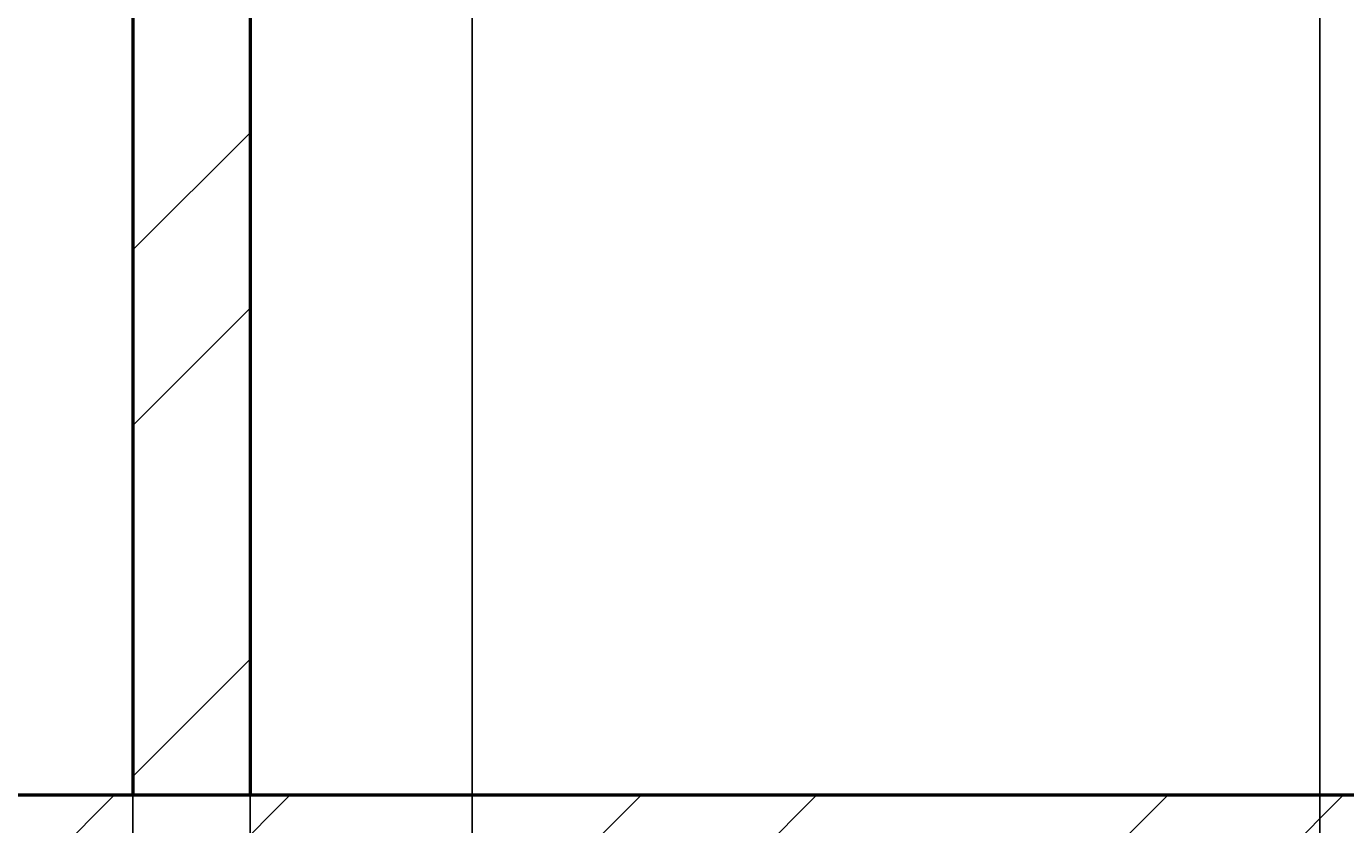
# Model space of a CAD drawing. Units: inches. Extents: x 2812 to 3051, y 1398 to 1659.
# Tile 50 of 65: x 2878 to 2911, y 1559 to 1579. Entities that reach past the tile are written whole.
import ezdxf

# ---------------------------------------------------------------- set-up
doc = ezdxf.new("R2010")
doc.units = ezdxf.units.IN
for name, color, linetype, lineweight in [('A-ANNO-DIMS', 2, 'Continuous', 18), ('S-CONC', 7, 'Continuous', 50), ('S-CONC-PATT', 8, 'Continuous', 18)]:
    doc.layers.add(name, color=color, linetype=linetype, lineweight=lineweight)
doc.styles.get("Standard").update_dxf_attribs({"font": 'arial.ttf'})
doc.dimstyles.get("Standard").update_dxf_attribs({"dimtxt": 0.18, "dimasz": 0.18, "dimexe": 0.18, "dimexo": 0.0625, "dimgap": 0.09, "dimtad": 0, "dimtih": 1, "dimtoh": 1, "dimdec": 4, "dimzin": 0, "dimdsep": 46, "dimtxsty": 'Standard', "dimcen": 0.09, "dimadec": 0, "dimazin": 0, "dimtfac": 1, "dimtdec": 4, "dimtofl": 0, "dimtmove": 0, "dimatfit": 3, "dimfxl": 1, "dimtolj": 1, "dimtzin": 0, "dimarcsym": 0})

# ---------------------------------------------------------------- blocks, each defined once
blk = doc.blocks.new('*D29')
at = {"layer": 'A-ANNO-DIMS', "color": 0, "lineweight": -2, "transparency": 16777216}
for p, q in [((2910.742, 1598.757), (2910.742, 1397.505)), ((2883.385, 1559.757), (2883.385, 1397.505)), ((2883.565, 1397.685), (2896.598, 1397.685)), ((2910.562, 1397.685), (2897.528, 1397.685))]:
    blk.add_line(p, q, dxfattribs=at)
at = {"layer": 'A-ANNO-DIMS', "color": 0, "transparency": 16777216}
for points in [[(2883.565, 1397.715), (2883.565, 1397.655), (2883.385, 1397.685)], [(2910.562, 1397.715), (2910.562, 1397.655), (2910.742, 1397.685)]]:
    blk.add_solid(points, dxfattribs=at)
at = {"layer": 'Defpoints', "color": 0, "transparency": 16777216}
for p in [(2910.742, 1598.82), (2883.385, 1559.82), (2910.742, 1397.685)]:
    blk.add_point(p, dxfattribs=at)
at = {"layer": 'A-ANNO-DIMS', "color": 0, "transparency": 16777216, "insert": (2897.063, 1397.685), "char_height": 0.18, "attachment_point": 5}
blk.add_mtext('\\A1;27.357', dxfattribs=at)
blk = doc.blocks.new('*D37')
at = {"layer": 'A-ANNO-DIMS', "color": 0, "lineweight": -2, "transparency": 16777216}
for p, q in [((2910.679, 1598.82), (2811.806, 1598.82)), ((2811.986, 1598.64), (2811.986, 1579.502)), ((2811.986, 1560), (2811.986, 1579.138)), ((2883.322, 1559.82), (2811.806, 1559.82))]:
    blk.add_line(p, q, dxfattribs=at)
at = {"layer": 'A-ANNO-DIMS', "color": 0, "transparency": 16777216}
for points in [[(2811.956, 1598.64), (2812.016, 1598.64), (2811.986, 1598.82)], [(2811.956, 1560), (2812.016, 1560), (2811.986, 1559.82)]]:
    blk.add_solid(points, dxfattribs=at)
at = {"layer": 'Defpoints', "color": 0, "transparency": 16777216}
for p in [(2811.986, 1598.82), (2910.742, 1598.82), (2883.385, 1559.82)]:
    blk.add_point(p, dxfattribs=at)
at = {"layer": 'A-ANNO-DIMS', "color": 0, "transparency": 16777216, "insert": (2811.986, 1579.32), "char_height": 0.18, "attachment_point": 5}
blk.add_mtext('\\A1;39', dxfattribs=at)
blk = doc.blocks.new('*D58')
at = {"layer": 'A-ANNO-DIMS', "color": 0, "lineweight": -2, "transparency": 16777216}
for p, q in [((2880.385, 1472.098), (2880.385, 1659.35)), ((2883.385, 1472.098), (2883.385, 1659.35)), ((2880.565, 1659.17), (2881.736, 1659.17)), ((2883.205, 1659.17), (2882.034, 1659.17))]:
    blk.add_line(p, q, dxfattribs=at)
at = {"layer": 'A-ANNO-DIMS', "color": 0, "transparency": 16777216}
for points in [[(2880.565, 1659.2), (2880.565, 1659.14), (2880.385, 1659.17)], [(2883.205, 1659.2), (2883.205, 1659.14), (2883.385, 1659.17)]]:
    blk.add_solid(points, dxfattribs=at)
at = {"layer": 'Defpoints', "color": 0, "transparency": 16777216}
for p in [(2883.385, 1659.17), (2880.385, 1472.035), (2883.385, 1472.035)]:
    blk.add_point(p, dxfattribs=at)
at = {"layer": 'A-ANNO-DIMS', "color": 0, "transparency": 16777216, "insert": (2881.885, 1659.17), "char_height": 0.18, "attachment_point": 5}
blk.add_mtext('\\A1;3', dxfattribs=at)
blk = doc.blocks.new('*D59')
at = {"layer": 'A-ANNO-DIMS', "color": 0, "lineweight": -2, "transparency": 16777216}
for p, q in [((2883.385, 1452.098), (2883.385, 1659.35)), ((2889.058, 1467.465), (2889.058, 1659.35)), ((2883.565, 1659.17), (2885.828, 1659.17)), ((2888.878, 1659.17), (2886.615, 1659.17))]:
    blk.add_line(p, q, dxfattribs=at)
at = {"layer": 'A-ANNO-DIMS', "color": 0, "transparency": 16777216}
for points in [[(2883.565, 1659.2), (2883.565, 1659.14), (2883.385, 1659.17)], [(2888.878, 1659.2), (2888.878, 1659.14), (2889.058, 1659.17)]]:
    blk.add_solid(points, dxfattribs=at)
at = {"layer": 'Defpoints', "color": 0, "transparency": 16777216}
for p in [(2889.058, 1659.17), (2889.058, 1467.402), (2883.385, 1452.035)]:
    blk.add_point(p, dxfattribs=at)
at = {"layer": 'A-ANNO-DIMS', "color": 0, "transparency": 16777216, "insert": (2886.221, 1659.17), "char_height": 0.18, "attachment_point": 5}
blk.add_mtext('\\A1;5.673', dxfattribs=at)

msp = doc.modelspace()

# ---------------------------------------------------------------- hatches: boundary and pattern name
at = {"layer": 'S-CONC-PATT'}
h = msp.add_hatch(dxfattribs=at)
h.set_pattern_fill('ANSI32', color=256)
h.paths.add_polyline_path([(3027.3849, 1646.82), (2835.3849, 1646.82), (2835.3849, 1603.2296), (2844.3849, 1603.2296), (2844.3849, 1637.82), (3018.3849, 1637.82), (3018.3849, 1602.5441), (3027.3849, 1602.5441)])
h.paths.add_polyline_path([(2844.3849, 1594.2296), (2835.3849, 1594.2296), (2835.3849, 1550.82), (3027.3849, 1550.82), (3027.3849, 1593.5441), (3018.3849, 1593.5441), (3018.3849, 1559.82), (2844.3849, 1559.82)])
h.paths.add_polyline_path([(2844.3849, 1482.0354), (2835.3849, 1482.0354), (2835.3849, 1463.4959), (2844.3849, 1463.4959)])
h.paths.add_polyline_path([(2844.3849, 1461.4959), (2835.3849, 1461.4959), (2835.3849, 1416.0354), (2844.3849, 1416.0354)])
h.paths.add_polyline_path([(3027.3849, 1482.0354), (3018.3849, 1482.0354), (3018.3849, 1463.2854), (3027.3849, 1463.2854)])
h.paths.add_polyline_path([(3027.3849, 1461.2854), (3018.3849, 1461.2854), (3018.3849, 1416.0354), (3027.3849, 1416.0354)])
h.paths.add_polyline_path([(2961.3849, 1448.4738), (2952.3849, 1448.4738), (2952.3849, 1416.0354), (2961.3849, 1416.0354)])
h.paths.add_polyline_path([(2961.3849, 1462.3026), (2952.3849, 1462.3026), (2952.3849, 1450.4738), (2961.3849, 1450.4738)])
h.paths.add_polyline_path([(2961.3849, 1472.0354), (2952.3849, 1472.0354), (2952.3849, 1462.3026), (2961.3849, 1462.3026)])
h = msp.add_hatch(dxfattribs=at)
h.set_pattern_fill('ANSI32', color=256)
h.paths.add_polyline_path([(2961.3849, 1637.82), (2952.3849, 1637.82), (2952.3849, 1603.2541), (2961.3849, 1603.2541)])
h.paths.add_polyline_path([(2961.3849, 1594.2541), (2952.3849, 1594.2541), (2952.3849, 1559.82), (2961.3849, 1559.82)])
h.paths.add_polyline_path([(2883.3849, 1637.82), (2880.3849, 1637.82), (2880.3849, 1559.82), (2883.3849, 1559.82)])

# ---------------------------------------------------------------- linework, layer by layer
at = {"layer": 'S-CONC'}
for p, q in [((2880.3849, 1637.82), (2880.3849, 1559.82)), ((2883.3849, 1637.82), (2883.3849, 1559.82)), ((2844.3849, 1559.82), (3018.3849, 1559.82))]:
    msp.add_line(p, q, dxfattribs=at)

# ---------------------------------------------------------------- dimensions: what is measured, and where the dimension line sits
at = {"layer": 'A-ANNO-DIMS'}
for base, p1, p2, override, picture, middle in [((2883.3849, 1659.17), (2880.3849, 1472.0354), (2883.3849, 1472.0354), {"dimdec": 0, "dimlfac": 1, "dimrnd": 0, "dimzin": 0, "dimdsep": 46, "dimlunit": 2}, '*D58', (2881.8849, 1659.17)), ((2889.0577, 1659.17), (2883.3849, 1452.0354), (2889.0577, 1467.4024), {"dimdec": 3, "dimlfac": 1, "dimrnd": 0, "dimzin": 0, "dimdsep": 46, "dimlunit": 2}, '*D59', (2886.2213, 1659.17)), ((2910.7415, 1397.6854), (2883.3849, 1559.82), (2910.7415, 1598.82), {"dimdec": 3, "dimlfac": 1, "dimrnd": 0, "dimzin": 0, "dimdsep": 46, "dimlunit": 2}, '*D29', (2897.0632, 1397.6854))]:
    dim = msp.add_linear_dim(base=base, p1=p1, p2=p2, dimstyle='Standard', override=override, dxfattribs=at)
    dim.commit()
    dim.dimension.update_dxf_attribs({"geometry": picture, "text_midpoint": middle})
dim = msp.add_linear_dim(base=(2811.9855, 1598.82), p1=(2883.3849, 1559.82), p2=(2910.7415, 1598.82), angle=90, dimstyle='Standard', override={"dimdec": 0, "dimlfac": 1, "dimrnd": 0, "dimzin": 0, "dimdsep": 46, "dimlunit": 2}, dxfattribs=at)
dim.commit()
dim.dimension.update_dxf_attribs({"geometry": '*D37', "text_midpoint": (2811.9855, 1579.32)})

doc.saveas('drawing.dxf')
